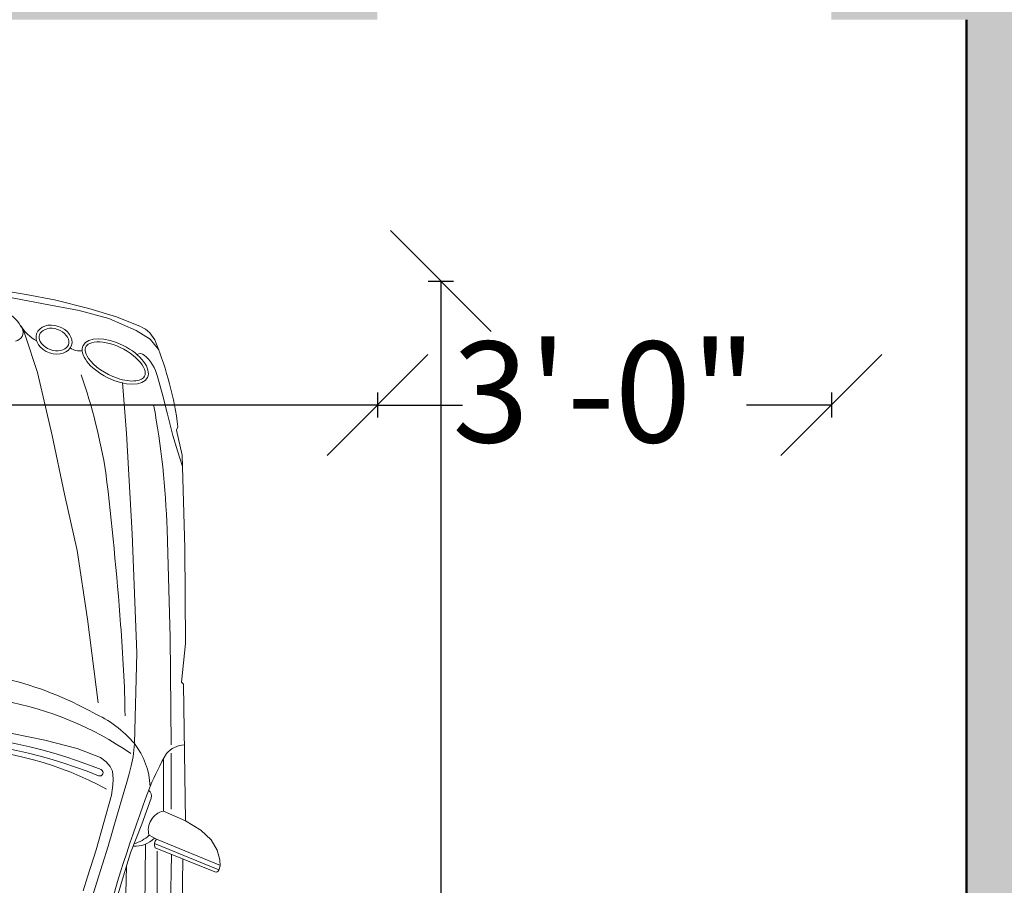
# Model space of a CAD drawing. Units: inches. Extents: x 3121 to 3511, y 1323 to 1998.
# Tile 5 of 10: x 3244 to 3322, y 1470 to 1539. Entities that reach past the tile are written whole.
import ezdxf

# ---------------------------------------------------------------- set-up
doc = ezdxf.new("R2010")
doc.units = ezdxf.units.IN
for name, color, linetype, lineweight in [('0_Equip', 250, 'Continuous', 13), ('A-ANNO-DIMS', 2, 'Continuous', 18), ('A-WALL', 7, 'Continuous', 50), ('A-WALL-PATT', 3, 'Continuous', 13)]:
    doc.layers.add(name, color=color, linetype=linetype, lineweight=lineweight)
doc.styles.get("Standard").update_dxf_attribs({"font": 'arial.ttf'})
doc.dimstyles.new('ISO-25', dxfattribs={"dimtxt": 8, "dimasz": 8, "dimexe": 1, "dimexo": 1, "dimtad": 0, "dimtih": 1, "dimtoh": 1, "dimlunit": 3, "dimtxsty": 'Standard', "dimblk": 'OBLIQUE', "dimcen": 2.5, "dimclrt": 1, "dimadec": 0, "dimazin": 0, "dimtfac": 1, "dimtmove": 0, "dimatfit": 3, "dimfxl": 1, "dimfxlon": 1, "dimarcsym": 0})

# ---------------------------------------------------------------- blocks, each defined once
blk = doc.blocks.new('A$C4C7B54D1')
at = {"layer": '0_Equip', "ltscale": 0.1}
for p, q in [((-0.4338, 2.6505), (-0.3394, 2.6343)), ((-0.4376, 2.6343), (-0.284, 2.6045)), ((-0.3394, 2.6343), (-0.2477, 2.6168)), ((-0.284, 2.6045), (-0.1689, 2.5829)), ((-0.2477, 2.6168), (-0.1371, 2.5898)), ((-0.1689, 2.5829), (-0.0725, 2.557)), ((-0.1371, 2.5898), (-0.0481, 2.5628)), ((-0.0725, 2.557), (0.0153, 2.5181)), ((-0.0481, 2.5628), (0.0288, 2.5318)), ((0.0153, 2.5181), (0.06, 2.4907)), ((-0.343, 2.5037), (-0.3027, 2.3827)), ((0.06, 2.4907), (0.0879, 2.4562)), ((-0.3027, 2.3827), (-0.2552, 2.1797)), ((-0.0163, 2.1869), (-0.0293, 2.3511)), ((0.084, 2.3701), (0.1016, 2.308)), ((0.1016, 2.308), (0.1164, 2.2486)), ((0.1164, 2.2486), (0.1336, 2.1795)), ((0.1499, 2.2082), (0.1457, 2.1976)), ((0.1457, 2.1976), (0.1637, 2.1169)), ((-0.2552, 2.1797), (-0.2164, 1.9911)), ((0.0024, 1.863), (-0.0163, 2.1869)), ((0.1336, 2.1795), (0.1484, 2.1304)), ((0.1484, 2.1304), (0.1647, 2.0798)), ((0.1637, 2.1169), (0.1722, 1.8165)), ((-0.2164, 1.9911), (-0.1746, 1.8097)), ((0.1147, 1.8774), (0.1247, 1.5304)), ((0.0168, 1.48), (0.0024, 1.863)), ((-0.1746, 1.8097), (-0.1415, 1.588)), ((0.1722, 1.8165), (0.1743, 1.5098)), ((-0.1415, 1.588), (-0.107, 1.3187)), ((0.1247, 1.5304), (0.1276, 1.1834)), ((0.1743, 1.5098), (0.1616, 1.3846)), ((0.0097, 1.1868), (0.0168, 1.48)), ((0.1616, 1.3846), (0.1679, 1.3782)), ((0.1679, 1.3782), (0.1739, 0.9375)), ((-0.3847, 1.22), (-0.279, 1.1976)), ((-0.279, 1.1976), (-0.1751, 1.1716)), ((0.0052, 1.1447), (0.0097, 1.1868)), ((-0.1751, 1.1716), (-0.0999, 1.142)), ((-0.0011, 1.1151), (0.0052, 1.1447)), ((0.128, 1.1562), (0.128, 0.9761)), ((-0.0999, 1.142), (-0.0811, 1.1286)), ((-0.0811, 1.1286), (-0.0685, 1.1133)), ((-0.0685, 1.1133), (-0.0614, 1.0981)), ((-0.0073, 1.0892), (-0.0011, 1.1151)), ((0.1038, 1.139), (0.1038, 0.9693)), ((-0.0614, 1.0981), (-0.0587, 1.0739)), ((-0.0145, 1.0623), (-0.0073, 1.0892)), ((-0.0596, 1.0533), (-0.0646, 1.0211)), ((-0.0587, 1.0739), (-0.0596, 1.0533)), ((-0.027, 1.0229), (-0.0145, 1.0623)), ((-0.0646, 1.0211), (-0.1139, 0.8446)), ((-0.0449, 0.961), (-0.027, 1.0229)), ((0.0635, 1.011), (0.0331, 0.9277)), ((-0.0754, 0.8562), (-0.0449, 0.961)), ((0.1739, 0.9375), (0.1032, 0.9696)), ((0.0331, 0.9277), (-0.0028, 0.8345)), ((0.1739, 0.9375), (0.2232, 0.908)), ((0.0566, 0.8914), (0.0807, 0.8786)), ((0.2232, 0.908), (0.2574, 0.8764)), ((0.0322, -0.0735), (0.0457, 0.863)), ((0.074, 0.865), (0.2816, 0.7802)), ((0.0807, 0.8786), (0.2867, 0.7945)), ((0.2574, 0.8764), (0.2767, 0.8432)), ((-0.1139, 0.8446), (-0.1417, 0.7577)), ((-0.1112, 0.7406), (-0.0754, 0.8562)), ((-0.0028, 0.8345), (-0.0287, 0.7503)), ((0.0759, 0.8512), (0.269, 0.7738)), ((0.0824, 0.8406), (0.0842, 0.484)), ((0.1292, 0.8299), (0.111, -0.138)), ((0.2767, 0.8432), (0.2853, 0.8127)), ((0.1658, 0.8152), (0.145, -0.6171)), ((0.2853, 0.8127), (0.2863, 0.7934)), ((-0.0162, 0.792), (-0.0361, -0.045)), ((0.2863, 0.7934), (0.2813, 0.7794)), ((-0.1417, 0.7577), (-0.156, 0.7129)), ((-0.1363, 0.66), (-0.1112, 0.7406)), ((-0.0287, 0.7503), (-0.0484, 0.6849))]:
    blk.add_line(p, q, dxfattribs=at)
for centre, radius, start, end in [((-0.4714, 2.461), 0.1353, 28.7147, 59.1631), ((-0.3785, 2.5126), 0.029, 278.279, 27.3962), ((-0.236, 2.6098), 0.1432, 211.8169, 240.8436), ((-0.4714, 2.461), 0.1353, 18.4111, 28.7147), ((-0.0123, 2.4422), 0.0986, 22.4887, 65.4055), ((-0.9791, 2.0579), 1.139, 7.5797, 21.7436), ((-0.1672, 2.5028), 0.0501, 233.2932, 279.4552), ((0.0285, 2.4259), 0.0184, 45.9796, 125.1948), ((-0.043, 2.3394), 0.1306, 13.5776, 49.7916), ((-2.0015, 1.746), 1.9445, 9.2981, 18.8883), ((-2.5715, 1.7918), 2.6875, 1.8245, 10.4459), ((-10.7169, 0.7813), 10.7109, 4.22626, 6.85742), ((-4.4136, 1.2089), 4.3935, 0.8876, 4.7233), ((-0.6653, 0.3109), 1.1158, 60.8852, 76.3449), ((-0.5976, 0.2949), 1.0461, 55.3038, 79.8165), ((-0.2711, 0.9494), 0.3676, 40.2153, 66.1489), ((-0.7157, -0.4312), 1.6538, 68.0714, 90.3446), ((-0.7157, -0.4312), 1.6329, 68.0714, 90.3446), ((-0.1807, 1.0395), 0.2408, 2.2254, 37.7282), ((0.1747, 1.102), 0.0813, 92.9311, 139.722), ((-0.6014, 0.0855), 1.0875, 61.3987, 88.1108), ((0.8964, 0.6968), 0.9076, 149.7096, 157.176), ((-0.102, 1.0932), 0.0105, 248.0714, 68.0714), ((5.1546, -0.8606), 5.4408, 159.4549, 164.9096), ((0.0373, 1.0171), 0.0269, 346.8936, 47.6723), ((0.1171, 0.9084), 0.0628, 102.7652, 195.6717), ((-0.0281, 0.9849), 0.1262, 286.919, 312.1713), ((0.0117, 0.9441), 0.0879, 266.0708, 315.2068), ((0.0982, 0.8614), 0.0245, 135.4886, 204.5013), ((0.2725, 0.7825), 0.00941, 248.1384, 340.354)]:
    blk.add_arc(centre, radius, start, end, dxfattribs=at)
at = {"layer": '0_Equip', "ltscale": 0.1, "extrusion": (0, 0, -1)}
for centre, major_axis, ratio in [((-0.2497, 2.4892), (-0.0562, 0.0189), 0.759763), ((-0.0523, 2.4187), (0.1036, -0.0518), 0.497493)]:
    blk.add_ellipse(centre, major_axis=major_axis, ratio=ratio, dxfattribs=at)
at = {"layer": '0_Equip', "ltscale": 0.1}
for points, knots in [([(-0.2965, 2.5048), (-0.2917, 2.5191), (-0.2703, 2.5294), (-0.2231, 2.5198), (-0.2033, 2.5001), (-0.2003, 2.4679), (-0.2141, 2.4539), (-0.2592, 2.4512), (-0.2858, 2.4658), (-0.2981, 2.4906), (-0.2987, 2.4983), (-0.2965, 2.5048)], [0, 0, 0, 0, 1.408119, 1.408119, 2.816238, 2.816238, 4.224358, 4.224358, 5.632477, 5.632477, 6.283185, 6.283185, 6.283185, 6.283185]), ([(0.0424, 2.3714), (0.0388, 2.3641), (0.0295, 2.3581), (-0.0022, 2.3543), (-0.0236, 2.3571), (-0.0834, 2.3771), (-0.1216, 2.404), (-0.152, 2.4483), (-0.152, 2.4626), (-0.1343, 2.4801), (-0.1108, 2.4849), (-0.0524, 2.4733), (-0.019, 2.4577), (0.0303, 2.4186), (0.0443, 2.3954), (0.0445, 2.3774), (0.0438, 2.3742), (0.0424, 2.3714)], [0, 0, 0, 0, 0.646556, 0.646556, 1.293113, 1.293113, 2.410172, 2.410172, 3.309931, 3.309931, 4.20969, 4.20969, 5.109449, 5.109449, 6.031285, 6.031285, 6.283185, 6.283185, 6.283185, 6.283185])]:
    blk.add_open_spline(points, degree=3, knots=knots, dxfattribs=at)
blk = doc.blocks.new('_Oblique')
at = {"color": 0, "linetype": 'ByBlock', "lineweight": -2}
blk.add_line((-0.5, -0.5), (0.5, 0.5), dxfattribs=at)
blk = doc.blocks.new('*D31')
at = {"layer": 'A-ANNO-DIMS', "color": 0, "lineweight": -2, "transparency": 16777216}
for p, q in [((3276.231, 1518.068), (3278.231, 1518.068)), ((3277.231, 1518.068), (3277.231, 1464.563)), ((3277.231, 1401.535), (3277.231, 1455.04)), ((3276.231, 1401.535), (3278.231, 1401.535))]:
    blk.add_line(p, q, dxfattribs=at)
at = {"layer": 'Defpoints', "color": 0, "transparency": 16777216}
for p in [(3259.751, 1518.068), (3277.231, 1518.068), (3259.751, 1401.535)]:
    blk.add_point(p, dxfattribs=at)
at = {"layer": 'A-ANNO-DIMS', "color": 0, "lineweight": -2, "transparency": 16777216, "xscale": 8, "yscale": 8, "zscale": 8}
for p, rotation in [((3277.231, 1518.068), 90), ((3277.231, 1401.535), 270)]:
    blk.add_blockref('_Oblique', p, dxfattribs=dict(at, rotation=rotation))
at = {"layer": 'A-ANNO-DIMS', "color": 1, "transparency": 16777216, "insert": (3277.231, 1459.801), "char_height": 8, "attachment_point": 5}
blk.add_mtext('CAR 9\'-8 1/2"', dxfattribs=at)
blk = doc.blocks.new('*D53')
at = {"layer": 'A-ANNO-DIMS', "color": 0, "lineweight": -2, "transparency": 16777216}
for p, q in [((3274.023, 1336.367), (3274.023, 1334.367)), ((3310.023, 1336.367), (3310.023, 1334.367)), ((3274.023, 1335.367), (3280.768, 1335.367)), ((3310.023, 1335.367), (3303.278, 1335.367))]:
    blk.add_line(p, q, dxfattribs=at)
at = {"layer": 'Defpoints', "color": 0, "transparency": 16777216}
for p in [(3274.023, 1946.784), (3310.023, 1946.784), (3310.023, 1335.367)]:
    blk.add_point(p, dxfattribs=at)
at = {"layer": 'A-ANNO-DIMS', "color": 0, "lineweight": -2, "transparency": 16777216, "xscale": 8, "yscale": 8, "zscale": 8, "rotation": 180}
blk.add_blockref('_Oblique', (3274.023, 1335.367), dxfattribs=at)
at = {"layer": 'A-ANNO-DIMS', "color": 0, "lineweight": -2, "transparency": 16777216, "xscale": 8, "yscale": 8, "zscale": 8}
blk.add_blockref('_Oblique', (3310.023, 1335.367), dxfattribs=at)
at = {"layer": 'A-ANNO-DIMS', "color": 1, "transparency": 16777216, "insert": (3292.023, 1335.367), "char_height": 8, "attachment_point": 5}
blk.add_mtext('3\'-0"', dxfattribs=at)
blk = doc.blocks.new('*D54')
at = {"layer": 'A-ANNO-DIMS', "color": 0, "lineweight": -2, "transparency": 16777216}
for p, q in [((3310.023, 1336.367), (3310.023, 1334.367)), ((3334.156, 1336.367), (3334.156, 1334.367)), ((3310.023, 1335.367), (3310.763, 1335.367)), ((3334.156, 1335.367), (3333.416, 1335.367))]:
    blk.add_line(p, q, dxfattribs=at)
at = {"layer": 'Defpoints', "color": 0, "transparency": 16777216}
for p in [(3310.023, 1946.784), (3334.156, 1946.784), (3334.156, 1335.367)]:
    blk.add_point(p, dxfattribs=at)
at = {"layer": 'A-ANNO-DIMS', "color": 0, "lineweight": -2, "transparency": 16777216, "xscale": 8, "yscale": 8, "zscale": 8, "rotation": 180}
blk.add_blockref('_Oblique', (3310.023, 1335.367), dxfattribs=at)
at = {"layer": 'A-ANNO-DIMS', "color": 0, "lineweight": -2, "transparency": 16777216, "xscale": 8, "yscale": 8, "zscale": 8}
blk.add_blockref('_Oblique', (3334.156, 1335.367), dxfattribs=at)
at = {"layer": 'A-ANNO-DIMS', "color": 1, "transparency": 16777216, "insert": (3322.089, 1335.367), "char_height": 8, "attachment_point": 5}
blk.add_mtext('2\'-0"', dxfattribs=at)
blk = doc.blocks.new('*D58')
at = {"layer": 'A-ANNO-DIMS', "color": 0, "lineweight": -2, "transparency": 16777216}
for p, q in [((3209.892, 1985.334), (3209.892, 1987.334)), ((3311.328, 1985.334), (3311.328, 1987.334)), ((3209.892, 1986.334), (3240.026, 1986.334)), ((3311.328, 1986.334), (3281.194, 1986.334))]:
    blk.add_line(p, q, dxfattribs=at)
at = {"layer": 'Defpoints', "color": 0, "transparency": 16777216}
for p in [(3311.328, 1986.334), (3209.892, 1424.784), (3311.328, 1424.784)]:
    blk.add_point(p, dxfattribs=at)
at = {"layer": 'A-ANNO-DIMS', "color": 0, "lineweight": -2, "transparency": 16777216, "xscale": 8, "yscale": 8, "zscale": 8, "rotation": 180}
blk.add_blockref('_Oblique', (3209.892, 1986.334), dxfattribs=at)
at = {"layer": 'A-ANNO-DIMS', "color": 0, "lineweight": -2, "transparency": 16777216, "xscale": 8, "yscale": 8, "zscale": 8}
blk.add_blockref('_Oblique', (3311.328, 1986.334), dxfattribs=at)
at = {"layer": 'A-ANNO-DIMS', "color": 1, "transparency": 16777216, "insert": (3260.61, 1986.334), "char_height": 8, "attachment_point": 5}
blk.add_mtext('8\'-5 1/2"', dxfattribs=at)
blk = doc.blocks.new('*D59')
at = {"layer": 'A-ANNO-DIMS', "color": 0, "lineweight": -2, "transparency": 16777216}
for p, q in [((3318.918, 1336.367), (3318.918, 1334.367)), ((3370.918, 1336.367), (3370.918, 1334.367)), ((3318.918, 1335.367), (3333.499, 1335.367)), ((3370.918, 1335.367), (3356.337, 1335.367))]:
    blk.add_line(p, q, dxfattribs=at)
at = {"layer": 'Defpoints', "color": 0, "transparency": 16777216}
for p in [(3318.918, 1752.226), (3370.918, 1748.784), (3370.918, 1335.367)]:
    blk.add_point(p, dxfattribs=at)
at = {"layer": 'A-ANNO-DIMS', "color": 0, "lineweight": -2, "transparency": 16777216, "xscale": 8, "yscale": 8, "zscale": 8, "rotation": 180}
blk.add_blockref('_Oblique', (3318.918, 1335.367), dxfattribs=at)
at = {"layer": 'A-ANNO-DIMS', "color": 0, "lineweight": -2, "transparency": 16777216, "xscale": 8, "yscale": 8, "zscale": 8}
blk.add_blockref('_Oblique', (3370.918, 1335.367), dxfattribs=at)
at = {"layer": 'A-ANNO-DIMS', "color": 1, "transparency": 16777216, "insert": (3344.918, 1335.367), "char_height": 8, "attachment_point": 5}
blk.add_mtext('4\'-4"', dxfattribs=at)
blk = doc.blocks.new('*D69')
at = {"layer": 'A-ANNO-DIMS', "color": 0, "lineweight": -2, "transparency": 16777216}
for p, q in [((3238.766, 1509.234), (3238.766, 1507.234)), ((3272.208, 1509.234), (3272.208, 1507.234)), ((3238.766, 1508.234), (3230.766, 1508.234)), ((3272.208, 1508.234), (3238.766, 1508.234))]:
    blk.add_line(p, q, dxfattribs=at)
at = {"layer": 'Defpoints', "color": 0, "transparency": 16777216}
for p in [(3238.766, 1538.784), (3272.208, 1538.784), (3238.766, 1508.234)]:
    blk.add_point(p, dxfattribs=at)
at = {"layer": 'A-ANNO-DIMS', "color": 0, "lineweight": -2, "transparency": 16777216, "xscale": 8, "yscale": 8, "zscale": 8, "rotation": 180}
blk.add_blockref('_Oblique', (3238.766, 1508.234), dxfattribs=at)
at = {"layer": 'A-ANNO-DIMS', "color": 0, "lineweight": -2, "transparency": 16777216, "xscale": 8, "yscale": 8, "zscale": 8}
blk.add_blockref('_Oblique', (3272.208, 1508.234), dxfattribs=at)
at = {"layer": 'A-ANNO-DIMS', "color": 1, "transparency": 16777216, "insert": (3210.119, 1508.234), "char_height": 8, "attachment_point": 5}
blk.add_mtext('2\'-9 1/2"', dxfattribs=at)
blk = doc.blocks.new('*D70')
at = {"layer": 'A-ANNO-DIMS', "color": 0, "lineweight": -2, "transparency": 16777216}
for p, q in [((3272.208, 1509.234), (3272.208, 1507.234)), ((3308.208, 1509.234), (3308.208, 1507.234)), ((3272.208, 1508.234), (3278.952, 1508.234)), ((3308.208, 1508.234), (3301.463, 1508.234))]:
    blk.add_line(p, q, dxfattribs=at)
at = {"layer": 'Defpoints', "color": 0, "transparency": 16777216}
for p in [(3272.208, 1538.784), (3308.208, 1538.784), (3272.208, 1508.234)]:
    blk.add_point(p, dxfattribs=at)
at = {"layer": 'A-ANNO-DIMS', "color": 0, "lineweight": -2, "transparency": 16777216, "xscale": 8, "yscale": 8, "zscale": 8, "rotation": 180}
blk.add_blockref('_Oblique', (3272.208, 1508.234), dxfattribs=at)
at = {"layer": 'A-ANNO-DIMS', "color": 0, "lineweight": -2, "transparency": 16777216, "xscale": 8, "yscale": 8, "zscale": 8}
blk.add_blockref('_Oblique', (3308.208, 1508.234), dxfattribs=at)
at = {"layer": 'A-ANNO-DIMS', "color": 1, "transparency": 16777216, "insert": (3290.208, 1508.234), "char_height": 8, "attachment_point": 5}
blk.add_mtext('3\'-0"', dxfattribs=at)
blk = doc.blocks.new('*D73')
at = {"layer": 'A-ANNO-DIMS', "color": 0, "lineweight": -2, "transparency": 16777216}
for p, q in [((3261.023, 1336.367), (3261.023, 1334.367)), ((3301.026, 1336.367), (3301.026, 1334.367)), ((3261.023, 1335.367), (3269.769, 1335.367)), ((3301.026, 1335.367), (3292.28, 1335.367))]:
    blk.add_line(p, q, dxfattribs=at)
at = {"layer": 'Defpoints', "color": 0, "transparency": 16777216}
for p in [(3261.023, 1739.784), (3301.026, 1739.784), (3301.026, 1335.367)]:
    blk.add_point(p, dxfattribs=at)
at = {"layer": 'A-ANNO-DIMS', "color": 0, "lineweight": -2, "transparency": 16777216, "xscale": 8, "yscale": 8, "zscale": 8, "rotation": 180}
blk.add_blockref('_Oblique', (3261.023, 1335.367), dxfattribs=at)
at = {"layer": 'A-ANNO-DIMS', "color": 0, "lineweight": -2, "transparency": 16777216, "xscale": 8, "yscale": 8, "zscale": 8}
blk.add_blockref('_Oblique', (3301.026, 1335.367), dxfattribs=at)
at = {"layer": 'A-ANNO-DIMS', "color": 1, "transparency": 16777216, "insert": (3281.024, 1335.367), "char_height": 8, "attachment_point": 5}
blk.add_mtext('3\'-4"', dxfattribs=at)

msp = doc.modelspace()

# ---------------------------------------------------------------- hatches: boundary and pattern name
at = {"layer": 'A-WALL-PATT'}
h = msp.add_hatch(color=256, dxfattribs=at)
h.dxf.hatch_style = 1
h.paths.add_polyline_path([(3274.023, 1955.784), (3189.918, 1955.784), (3189.918, 1910.219), (3198.918, 1910.219), (3198.918, 1946.784), (3259.023, 1946.784), (3259.023, 1921.61), (3261.023, 1921.61), (3261.023, 1946.784), (3274.023, 1946.784)])
h.paths.add_polyline_path([(3327.918, 1946.784), (3334.156, 1946.784), (3334.156, 1955.784), (3310.023, 1955.784), (3310.023, 1946.784), (3318.918, 1946.784), (3318.918, 1929.796), (3311.644, 1929.796), (3311.644, 1927.007), (3324.033, 1927.007), (3324.033, 1871.381), (3311.644, 1871.381), (3311.644, 1868.381), (3318.918, 1868.381), (3318.918, 1853.784), (3327.918, 1853.784)])
h.paths.add_polyline_path([(3456.918, 1955.784), (3384.562, 1955.784), (3384.562, 1946.784), (3447.918, 1946.784), (3447.918, 1877.779), (3456.918, 1877.779)])
h.paths.add_polyline_path([(3456.918, 1835.782), (3447.918, 1835.782), (3447.918, 1814.784), (3414.918, 1814.784), (3414.918, 1803.784), (3447.918, 1803.784), (3447.918, 1793.443), (3456.918, 1793.443)])
h.paths.add_polyline_path([(3456.918, 1558.434), (3447.918, 1558.434), (3447.918, 1547.784), (3375.918, 1547.784), (3375.918, 1598.784), (3378.918, 1598.784), (3378.918, 1602.284), (3375.918, 1602.284), (3375.918, 1674.284), (3369.918, 1674.284), (3369.918, 1547.784), (3364.418, 1547.784), (3364.418, 1538.784), (3447.918, 1538.784), (3447.918, 1512.628), (3456.918, 1512.628)])
h.paths.add_polyline_path([(3456.918, 1460.558), (3447.918, 1460.558), (3447.918, 1424.784), (3412.543, 1424.784), (3412.543, 1415.784), (3456.918, 1415.784)])
h.paths.add_polyline_path([(3358.149, 1424.784), (3322.918, 1424.784), (3322.918, 1538.784), (3328.418, 1538.784), (3328.418, 1547.784), (3308.208, 1547.784), (3308.208, 1538.784), (3318.918, 1538.784), (3318.918, 1424.784), (3311.328, 1424.784), (3311.328, 1415.784), (3358.149, 1415.784)])
h.paths.add_polyline_path([(3207.562, 1547.784), (3198.918, 1547.784), (3198.918, 1607.327), (3189.918, 1607.327), (3189.918, 1513.073), (3198.918, 1513.073), (3198.918, 1538.784), (3207.562, 1538.784)])
h.paths.add_polyline_path([(3198.918, 1461.548), (3189.918, 1461.548), (3189.918, 1415.784), (3209.892, 1415.784), (3209.892, 1424.784), (3198.918, 1424.784)])
h.paths.add_polyline_path([(3272.208, 1547.784), (3238.766, 1547.784), (3238.766, 1538.784), (3272.208, 1538.784)])
h.paths.add_polyline_path([(3261.023, 1748.784), (3198.918, 1748.784), (3198.918, 1768.387), (3189.918, 1768.387), (3189.918, 1692.279), (3198.918, 1692.279), (3198.918, 1739.784), (3261.023, 1739.784)])
h.paths.add_polyline_path([(3198.918, 1856.171), (3189.918, 1856.171), (3189.918, 1808.331), (3198.918, 1808.331), (3198.918, 1821.074), (3261.023, 1821.074), (3261.023, 1862.309), (3259.023, 1862.309), (3259.023, 1825.074), (3198.918, 1825.074)])

# ---------------------------------------------------------------- linework, layer by layer
at = {"layer": 'A-WALL'}
msp.add_line((3318.918, 1424.784), (3318.918, 1538.784), dxfattribs=at)

# ---------------------------------------------------------------- block references
at = {"layer": '0_Equip', "xscale": 24.59625072819005, "yscale": 24.59625072819005, "zscale": 24.59625072819005}
msp.add_blockref('A$C4C7B54D1', (3252.699, 1452.199), dxfattribs=at)

# ---------------------------------------------------------------- dimensions: what is measured, and where the dimension line sits
at = {"layer": 'A-ANNO-DIMS'}
for base, p1, p2, picture, middle in [((3311.328, 1986.334), (3209.892, 1424.784), (3311.328, 1424.784), '*D58', (3260.61, 1986.334)), ((3310.023, 1335.367), (3274.023, 1946.784), (3310.023, 1946.784), '*D53', (3292.023, 1335.367)), ((3334.156, 1335.367), (3310.023, 1946.784), (3334.156, 1946.784), '*D54', (3322.089, 1335.367)), ((3370.918, 1335.367), (3318.918, 1752.226), (3370.918, 1748.784), '*D59', (3344.918, 1335.367)), ((3301.026, 1335.367), (3261.023, 1739.784), (3301.026, 1739.784), '*D73', (3281.024, 1335.367))]:
    dim = msp.add_linear_dim(base=base, p1=p1, p2=p2, dimstyle='ISO-25', override={"dimdec": 1, "dimlfac": 1, "dimrnd": 0, "dimzin": 1, "dimdsep": 46, "dimlunit": 4, "dimfrac": 2}, dxfattribs=at)
    dim.commit()
    dim.dimension.update_dxf_attribs({"geometry": picture, "text_midpoint": middle})
for base, p1, p2, picture, middle in [((3238.766, 1508.234), (3272.208, 1538.784), (3238.766, 1538.784), '*D69', (3210.119, 1508.234)), ((3272.208, 1508.234), (3308.208, 1538.784), (3272.208, 1538.784), '*D70', (3290.208, 1508.234))]:
    dim = msp.add_linear_dim(base=base, p1=p1, p2=p2, angle=180, dimstyle='ISO-25', override={"dimdec": 1, "dimlfac": 1, "dimrnd": 0, "dimzin": 1, "dimdsep": 46, "dimlunit": 4, "dimfrac": 2}, dxfattribs=at)
    dim.commit()
    dim.dimension.update_dxf_attribs({"geometry": picture, "text_midpoint": middle})
dim = msp.add_linear_dim(base=(3277.231, 1518.068), p1=(3259.751, 1401.535), p2=(3259.751, 1518.068), angle=90, text='CAR <>', dimstyle='ISO-25', override={"dimdec": 1, "dimlfac": 1, "dimrnd": 0, "dimzin": 1, "dimdsep": 46, "dimlunit": 4, "dimfrac": 2}, dxfattribs=at)
dim.commit()
dim.dimension.update_dxf_attribs({"geometry": '*D31', "text_midpoint": (3277.231, 1459.801)})

doc.saveas('drawing.dxf')
